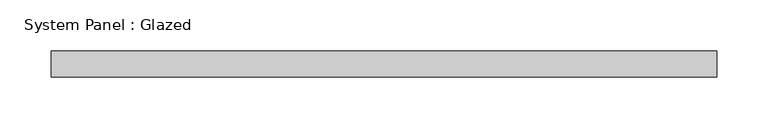
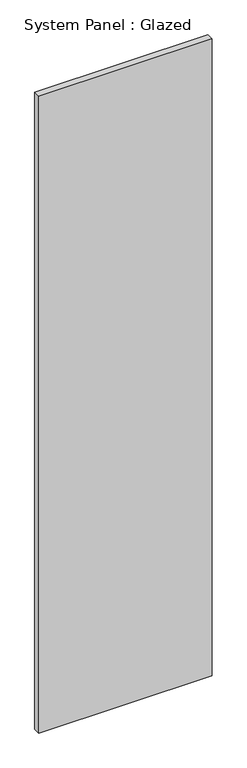
"""IFC4 building model written with IfcOpenShell, lengths in millimetres: plate geometry, System Panel : Glazed."""

from ifc_helpers import new_model, si_unit, origin, origin_with_axes, place, context, project, spatial, polyline, outline, extrude, source, transform, mapped, element, save


def system_panel_glazed_744525f6(model_context):
    return source(origin(), model_context, "Body", "SweptSolid", [
        extrude(outline(polyline([(323.85, 19.05), (-323.85, 19.05), (-323.85, 44.45), (323.85, 44.45), (323.85, 19.05)])), origin_with_axes(), (0.0, 0.0, 1.0), 2514.6),
    ])


if __name__ == "__main__":
    model = new_model("IFC4")
    model_context = context("Model", 3, world=origin())
    ifc_project = project(units=[si_unit("LENGTHUNIT", "METRE", prefix="MILLI")], contexts=[model_context])
    site = spatial("IfcSite", under=ifc_project)
    building = spatial("IfcBuilding", under=site)
    placement = place(None, origin())
    system_panel_glazed_shape = system_panel_glazed_744525f6(model_context)
    element("IfcPlate", 1, ObjectType="System Panel : Glazed", at=placement, inside=building, context=model_context, shape_type="MappedRepresentation", body=[
        mapped(system_panel_glazed_shape, transform((0.0, 0.0, 0.0), x_axis=(1.0, 0.0, 0.0), y_axis=(0.0, 1.0, 0.0), z_axis=(0.0, 0.0, 1.0))),
    ])
    save(model, "model.ifc")

# Revit data of these elements
# Type "System Panel : Glazed"
#   Construction Type Id = "GSP4R"
#   Analytic Construction = "1/8 in Pilkington single glazing"
#   Visual Light Transmittance = 0.9
#   Solar Heat Gain Coefficient = 0.86
#   Heat Transfer Coefficient (U) = 1.18115 BTU/(h·ft²·°F)
#   Define Thermal Properties by = 1
# Element 1 (IfcPlate, "System Panel : Glazed")
#   Materials on its faces: "Glass"
# Materials
#   "Glass": class "Glass", colour RGB 0 128 192, transparency 0.75, Description = "Soda Lime Glass", Cost = 0
